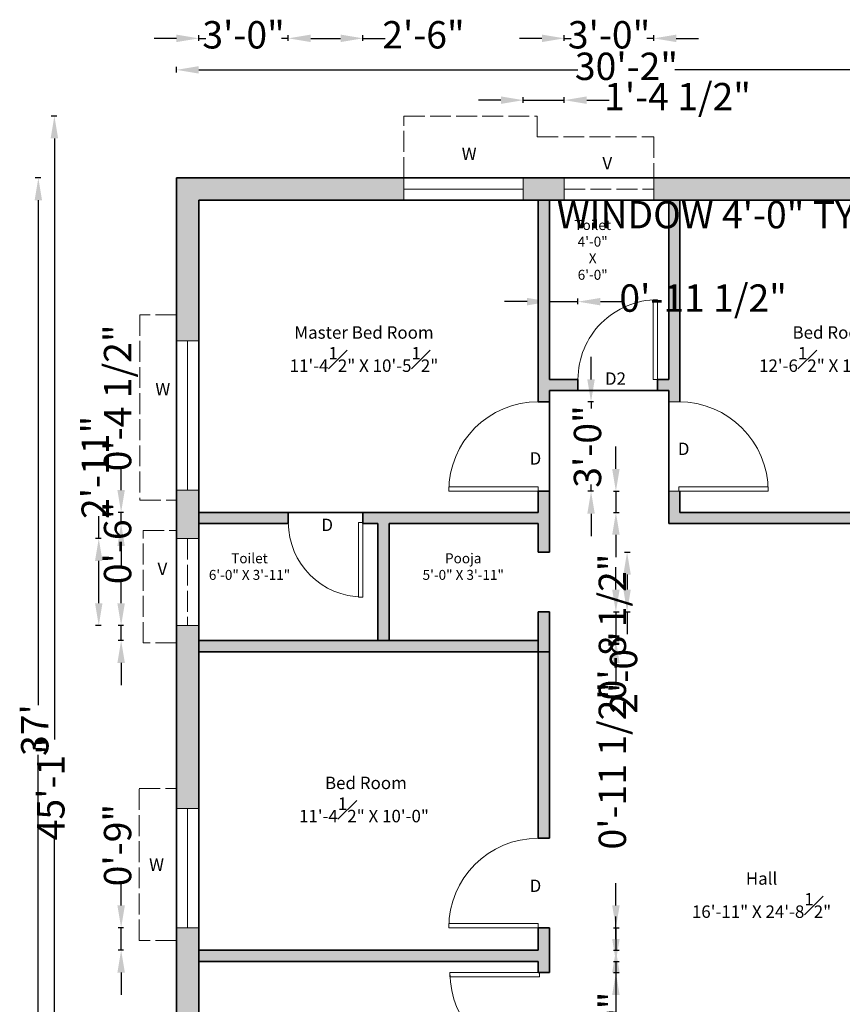
# Model space of a CAD drawing. Units: inches. Extents: x 2339 to 2848, y 489 to 1121.
# Tile 2 of 3: x 2339 to 2670, y 725 to 1121. Entities that reach past the tile are written whole.
import ezdxf

# ---------------------------------------------------------------- set-up
doc = ezdxf.new("R2010")
doc.units = ezdxf.units.IN
doc.linetypes.add('ACAD_ISO02W100', pattern=[15, 12, -3])
for name, color, linetype, lineweight in [('A-ANNO-DIMS', 2, 'Continuous', 18), ('A-ANNO-TEXT', 7, 'Continuous', 18), ('A-AREA-IDEN', 7, 'Continuous', 18), ('A-DOOR', 3, 'Continuous', 18), ('A-GLAZ', 4, 'Continuous', 18), ('A-GLAZ-VENT', 4, 'ACAD_ISO02W100', 18), ('A-ROOF-OVHD', 8, 'ACAD_ISO02W100', 13), ('A-WALL', 7, 'Continuous', 35)]:
    doc.layers.add(name, color=color, linetype=linetype, lineweight=lineweight)
doc.layers.add('A-WALL-PATT', color=18, linetype='Continuous', lineweight=13, true_color=0x000000)
doc.styles.get("Standard").update_dxf_attribs({"font": 'arial.ttf'})
doc.dimstyles.new('ISO-25', dxfattribs={"dimtxt": 11, "dimasz": 9, "dimexe": 1.25, "dimexo": 0.625, "dimtad": 0, "dimlunit": 4, "dimtxsty": 'Standard', "dimcen": 2.5, "dimadec": 0, "dimazin": 0, "dimtfac": 1, "dimtmove": 0, "dimatfit": 3, "dimfxl": 1, "dimfxlon": 1, "dimfrac": 1, "dimarcsym": 0})

# ---------------------------------------------------------------- blocks, each defined once
blk = doc.blocks.new('*U1')
for p, q in [((0, 0), (0, 4)), ((32, 0), (32, 4))]:
    blk.add_line(p, q)
blk.add_lwpolyline([(0, 0), (0, -32), (1.75, -32), (1.75, 0)], close=True)
blk.add_arc((0, 0), 32, 270, 0)
blk = doc.blocks.new('*U2')
for p, q in [((0, 0), (0, -4)), ((36, 0), (36, -4))]:
    blk.add_line(p, q)
blk.add_lwpolyline([(0, 0), (0, 36), (1.75, 36), (1.75, 0)], close=True)
blk.add_arc((0, 0), 36, 0, 90)
blk = doc.blocks.new('*U3')
for p, q in [((0, 0), (0, 4)), ((30, 0), (30, 4))]:
    blk.add_line(p, q)
blk.add_lwpolyline([(0, 0), (0, -30), (1.75, -30), (1.75, 0)], close=True)
blk.add_arc((0, 0), 30, 270, 0)
blk = doc.blocks.new('*D4')
at = {"layer": 'A-ANNO-DIMS', "color": 0, "lineweight": -2, "transparency": 16777216}
for p, q in [((2347.8, 1057.44), (2345.55, 1057.44)), ((2346.8, 1048.44), (2346.8, 845.39)), ((2346.8, 622.44), (2346.8, 825.48)), ((2347.8, 613.44), (2345.55, 613.44))]:
    blk.add_line(p, q, dxfattribs=at)
at = {"layer": 'A-ANNO-DIMS', "color": 0, "transparency": 16777216}
for points in [[(2345.3, 1048.44), (2348.3, 1048.44), (2346.8, 1057.44)], [(2345.3, 622.44), (2348.3, 622.44), (2346.8, 613.44)]]:
    blk.add_solid(points, dxfattribs=at)
at = {"layer": 'Defpoints', "color": 0, "transparency": 16777216}
for p in [(2402.35, 1057.44), (2346.8, 613.44), (2402.35, 613.44)]:
    blk.add_point(p, dxfattribs=at)
at = {"layer": 'A-ANNO-DIMS', "color": 0, "transparency": 16777216, "insert": (2346.8, 835.44), "char_height": 11, "attachment_point": 5, "rotation": 90}
blk.add_mtext("37'", dxfattribs=at)
blk = doc.blocks.new('*D6')
at = {"layer": 'A-ANNO-DIMS', "color": 0, "lineweight": -2, "transparency": 16777216}
for p, q in [((2402.35, 1099.88), (2402.35, 1102.13)), ((2411.35, 1100.88), (2563.83, 1100.88)), ((2755.35, 1100.88), (2602.86, 1100.88)), ((2764.35, 1099.88), (2764.35, 1102.13))]:
    blk.add_line(p, q, dxfattribs=at)
at = {"layer": 'A-ANNO-DIMS', "color": 0, "transparency": 16777216}
for points in [[(2411.35, 1102.38), (2411.35, 1099.38), (2402.35, 1100.88)], [(2755.35, 1102.38), (2755.35, 1099.38), (2764.35, 1100.88)]]:
    blk.add_solid(points, dxfattribs=at)
at = {"layer": 'Defpoints', "color": 0, "transparency": 16777216}
for p in [(2764.35, 1100.88), (2402.35, 1057.44), (2764.35, 1057.44)]:
    blk.add_point(p, dxfattribs=at)
at = {"layer": 'A-ANNO-DIMS', "color": 0, "transparency": 16777216, "insert": (2583.35, 1100.88), "char_height": 11, "attachment_point": 5}
blk.add_mtext('30\'-2"', dxfattribs=at)
blk = doc.blocks.new('WIN-48IN')
for p, q in [((0, 0), (0, 9)), ((48, 0), (48, 9)), ((0, 4.5), (48, 4.5))]:
    blk.add_line(p, q)
blk = doc.blocks.new('*D9')
at = {"layer": 'A-ANNO-DIMS', "color": 0, "lineweight": -2, "transparency": 16777216}
for p, q in [((2701.35, 1041.24), (2692.35, 1041.24)), ((2701.35, 1042.24), (2701.35, 1039.99)), ((2740.35, 1041.24), (2710.35, 1041.24)), ((2749.35, 1042.24), (2749.35, 1039.99))]:
    blk.add_line(p, q, dxfattribs=at)
at = {"layer": 'A-ANNO-DIMS', "color": 0, "transparency": 16777216}
for points in [[(2710.35, 1042.74), (2710.35, 1039.74), (2701.35, 1041.24)], [(2740.35, 1042.74), (2740.35, 1039.74), (2749.35, 1041.24)]]:
    blk.add_solid(points, dxfattribs=at)
at = {"layer": 'Defpoints', "color": 0, "transparency": 16777216}
for p in [(2701.35, 1048.44), (2749.35, 1048.44), (2701.35, 1041.24)]:
    blk.add_point(p, dxfattribs=at)
at = {"layer": 'A-ANNO-DIMS', "color": 0, "transparency": 16777216, "insert": (2622.12, 1041.24), "char_height": 11, "attachment_point": 5}
blk.add_mtext('WINDOW 4\'-0" TYP.', dxfattribs=at)
blk = doc.blocks.new('*D11')
at = {"layer": 'A-ANNO-DIMS', "color": 0, "lineweight": -2, "transparency": 16777216}
for p, q in [((2354.26, 1082.3), (2352.01, 1082.3)), ((2353.26, 1073.3), (2353.26, 831.61)), ((2353.26, 550.44), (2353.26, 792.13)), ((2354.26, 541.44), (2352.01, 541.44))]:
    blk.add_line(p, q, dxfattribs=at)
at = {"layer": 'A-ANNO-DIMS', "color": 0, "transparency": 16777216}
for points in [[(2351.76, 1073.3), (2354.76, 1073.3), (2353.26, 1082.3)], [(2351.76, 550.44), (2354.76, 550.44), (2353.26, 541.44)]]:
    blk.add_solid(points, dxfattribs=at)
at = {"layer": 'Defpoints', "color": 0, "transparency": 16777216}
for p in [(2353.26, 1082.3), (2493.85, 1082.3), (2402.35, 541.44)]:
    blk.add_point(p, dxfattribs=at)
at = {"layer": 'A-ANNO-DIMS', "color": 0, "transparency": 16777216, "insert": (2353.26, 811.87), "char_height": 11, "attachment_point": 5, "rotation": 90}
blk.add_mtext('45\'-1"', dxfattribs=at)
blk = doc.blocks.new('*D22')
at = {"layer": 'A-ANNO-DIMS', "color": 0, "lineweight": -2, "transparency": 16777216}
for p, q in [((2380.1, 764.94), (2380.1, 773.94)), ((2381.1, 755.94), (2378.85, 755.94)), ((2380.1, 746.94), (2380.1, 755.94)), ((2381.1, 746.94), (2378.85, 746.94)), ((2380.1, 737.94), (2380.1, 728.94))]:
    blk.add_line(p, q, dxfattribs=at)
at = {"layer": 'A-ANNO-DIMS', "color": 0, "transparency": 16777216}
for points in [[(2378.6, 764.94), (2381.6, 764.94), (2380.1, 755.94)], [(2378.6, 737.94), (2381.6, 737.94), (2380.1, 746.94)]]:
    blk.add_solid(points, dxfattribs=at)
at = {"layer": 'Defpoints', "color": 0, "transparency": 16777216}
for p in [(2380.1, 755.94), (2411.35, 755.94), (2411.35, 746.94)]:
    blk.add_point(p, dxfattribs=at)
at = {"layer": 'A-ANNO-DIMS', "color": 0, "transparency": 16777216, "insert": (2380.1, 789.18), "char_height": 11, "attachment_point": 5, "rotation": 90}
blk.add_mtext('0\'-9"', dxfattribs=at)
blk = doc.blocks.new('*D23')
at = {"layer": 'A-ANNO-DIMS', "color": 0, "lineweight": -2, "transparency": 16777216}
for p, q in [((2380.1, 886.44), (2380.1, 895.44)), ((2381.1, 877.44), (2378.85, 877.44)), ((2380.1, 871.44), (2380.1, 877.44)), ((2381.1, 871.44), (2378.85, 871.44)), ((2380.1, 862.44), (2380.1, 853.44))]:
    blk.add_line(p, q, dxfattribs=at)
at = {"layer": 'A-ANNO-DIMS', "color": 0, "transparency": 16777216}
for points in [[(2378.6, 886.44), (2381.6, 886.44), (2380.1, 877.44)], [(2378.6, 862.44), (2381.6, 862.44), (2380.1, 871.44)]]:
    blk.add_solid(points, dxfattribs=at)
at = {"layer": 'Defpoints', "color": 0, "transparency": 16777216}
for p in [(2380.1, 877.44), (2411.35, 877.44), (2411.35, 871.44)]:
    blk.add_point(p, dxfattribs=at)
at = {"layer": 'A-ANNO-DIMS', "color": 0, "transparency": 16777216, "insert": (2380.1, 910.68), "char_height": 11, "attachment_point": 5, "rotation": 90}
blk.add_mtext('0\'-6"', dxfattribs=at)
blk = doc.blocks.new('*D24')
at = {"layer": 'A-ANNO-DIMS', "color": 0, "lineweight": -2, "transparency": 16777216}
for p, q in [((2371.1, 912.44), (2371.1, 921.44)), ((2372.1, 912.44), (2369.85, 912.44)), ((2371.1, 886.44), (2371.1, 903.44)), ((2372.1, 877.44), (2369.85, 877.44))]:
    blk.add_line(p, q, dxfattribs=at)
at = {"layer": 'A-ANNO-DIMS', "color": 0, "transparency": 16777216}
for points in [[(2369.6, 903.44), (2372.6, 903.44), (2371.1, 912.44)], [(2369.6, 886.44), (2372.6, 886.44), (2371.1, 877.44)]]:
    blk.add_solid(points, dxfattribs=at)
at = {"layer": 'Defpoints', "color": 0, "transparency": 16777216}
for p in [(2371.1, 912.44), (2402.35, 912.44), (2402.35, 877.44)]:
    blk.add_point(p, dxfattribs=at)
at = {"layer": 'A-ANNO-DIMS', "color": 0, "transparency": 16777216, "insert": (2371.1, 941.05), "char_height": 11, "attachment_point": 5, "rotation": 90}
blk.add_mtext('2\'-11"', dxfattribs=at)
blk = doc.blocks.new('*D25')
at = {"layer": 'A-ANNO-DIMS', "color": 0, "lineweight": -2, "transparency": 16777216}
for p, q in [((2830.6, 991.94), (2832.85, 991.94)), ((2831.6, 982.94), (2831.6, 977.18)), ((2831.6, 940.94), (2831.6, 946.69)), ((2830.6, 931.94), (2832.85, 931.94))]:
    blk.add_line(p, q, dxfattribs=at)
at = {"layer": 'A-ANNO-DIMS', "color": 0, "transparency": 16777216}
for points in [[(2830.1, 982.94), (2833.1, 982.94), (2831.6, 991.94)], [(2830.1, 940.94), (2833.1, 940.94), (2831.6, 931.94)]]:
    blk.add_solid(points, dxfattribs=at)
at = {"layer": 'Defpoints', "color": 0, "transparency": 16777216}
for p in [(2411.35, 991.94), (2831.6, 991.94), (2411.35, 931.94)]:
    blk.add_point(p, dxfattribs=at)
at = {"layer": 'A-ANNO-DIMS', "color": 0, "transparency": 16777216, "insert": (2831.6, 961.94), "char_height": 11, "attachment_point": 5, "rotation": 90}
blk.add_mtext('5\'-0"', dxfattribs=at)
blk = doc.blocks.new('*D26')
at = {"layer": 'A-ANNO-DIMS', "color": 0, "lineweight": -2, "transparency": 16777216}
for p, q in [((2831.6, 1048.44), (2831.6, 1057.44)), ((2830.6, 1048.44), (2832.85, 1048.44)), ((2831.6, 1000.94), (2831.6, 1039.44)), ((2830.6, 991.94), (2832.85, 991.94))]:
    blk.add_line(p, q, dxfattribs=at)
at = {"layer": 'A-ANNO-DIMS', "color": 0, "transparency": 16777216}
for points in [[(2830.1, 1039.44), (2833.1, 1039.44), (2831.6, 1048.44)], [(2830.1, 1000.94), (2833.1, 1000.94), (2831.6, 991.94)]]:
    blk.add_solid(points, dxfattribs=at)
at = {"layer": 'Defpoints', "color": 0, "transparency": 16777216}
for p in [(2411.35, 1048.44), (2831.6, 1048.44), (2411.35, 991.94)]:
    blk.add_point(p, dxfattribs=at)
at = {"layer": 'A-ANNO-DIMS', "color": 0, "transparency": 16777216, "insert": (2831.6, 1085.72), "char_height": 11, "attachment_point": 5, "rotation": 90}
blk.add_mtext('4\'-8 1/2"', dxfattribs=at)
blk = doc.blocks.new('*D27')
at = {"layer": 'A-ANNO-DIMS', "color": 0, "lineweight": -2, "transparency": 16777216}
for p, q in [((2411.35, 511.19), (2411.35, 508.94)), ((2493.85, 511.19), (2493.85, 508.94)), ((2402.35, 510.19), (2393.35, 510.19)), ((2411.35, 510.19), (2420.23, 510.19)), ((2493.85, 510.19), (2484.96, 510.19)), ((2502.85, 510.19), (2511.85, 510.19))]:
    blk.add_line(p, q, dxfattribs=at)
at = {"layer": 'A-ANNO-DIMS', "color": 0, "transparency": 16777216}
for points in [[(2402.35, 511.69), (2402.35, 508.69), (2411.35, 510.19)], [(2502.85, 511.69), (2502.85, 508.69), (2493.85, 510.19)]]:
    blk.add_solid(points, dxfattribs=at)
at = {"layer": 'Defpoints', "color": 0, "transparency": 16777216}
for p in [(2411.35, 1048.44), (2493.85, 1048.44), (2493.85, 510.19)]:
    blk.add_point(p, dxfattribs=at)
at = {"layer": 'A-ANNO-DIMS', "color": 0, "transparency": 16777216, "insert": (2452.6, 510.19), "char_height": 11, "attachment_point": 5}
blk.add_mtext('6\'-10 1/2"', dxfattribs=at)
blk = doc.blocks.new('*D28')
at = {"layer": 'A-ANNO-DIMS', "color": 0, "lineweight": -2, "transparency": 16777216}
for p, q in [((2549.35, 1113.55), (2540.35, 1113.55)), ((2558.35, 1112.55), (2558.35, 1114.8)), ((2558.35, 1113.55), (2561.11, 1113.55)), ((2594.35, 1113.55), (2591.59, 1113.55)), ((2594.35, 1112.55), (2594.35, 1114.8)), ((2603.35, 1113.55), (2612.35, 1113.55))]:
    blk.add_line(p, q, dxfattribs=at)
at = {"layer": 'A-ANNO-DIMS', "color": 0, "transparency": 16777216}
for points in [[(2549.35, 1115.05), (2549.35, 1112.05), (2558.35, 1113.55)], [(2603.35, 1115.05), (2603.35, 1112.05), (2594.35, 1113.55)]]:
    blk.add_solid(points, dxfattribs=at)
at = {"layer": 'Defpoints', "color": 0, "transparency": 16777216}
for p in [(2594.35, 1113.55), (2558.35, 1057.44), (2594.35, 1057.44)]:
    blk.add_point(p, dxfattribs=at)
at = {"layer": 'A-ANNO-DIMS', "color": 0, "transparency": 16777216, "insert": (2576.35, 1113.55), "char_height": 11, "attachment_point": 5}
blk.add_mtext('3\'-0"', dxfattribs=at)
blk = doc.blocks.new('*D29')
at = {"layer": 'A-ANNO-DIMS', "color": 0, "lineweight": -2, "transparency": 16777216}
for p, q in [((2532.85, 1088.69), (2523.85, 1088.69)), ((2541.85, 1087.69), (2541.85, 1089.94)), ((2541.85, 1088.69), (2558.35, 1088.69)), ((2558.35, 1087.69), (2558.35, 1089.94)), ((2567.35, 1088.69), (2576.35, 1088.69))]:
    blk.add_line(p, q, dxfattribs=at)
at = {"layer": 'A-ANNO-DIMS', "color": 0, "transparency": 16777216}
for points in [[(2532.85, 1090.19), (2532.85, 1087.19), (2541.85, 1088.69)], [(2567.35, 1090.19), (2567.35, 1087.19), (2558.35, 1088.69)]]:
    blk.add_solid(points, dxfattribs=at)
at = {"layer": 'Defpoints', "color": 0, "transparency": 16777216}
for p in [(2558.35, 1088.69), (2541.85, 1057.44), (2558.35, 1057.44)]:
    blk.add_point(p, dxfattribs=at)
at = {"layer": 'A-ANNO-DIMS', "color": 0, "transparency": 16777216, "insert": (2603.89, 1088.69), "char_height": 11, "attachment_point": 5}
blk.add_mtext('1\'-4 1/2"', dxfattribs=at)
blk = doc.blocks.new('*D36')
at = {"layer": 'A-ANNO-DIMS', "color": 0, "lineweight": -2, "transparency": 16777216}
for p, q in [((2563.85, 511.19), (2563.85, 508.94)), ((2595.85, 511.19), (2595.85, 508.94)), ((2554.85, 510.19), (2545.85, 510.19)), ((2563.85, 510.19), (2564.51, 510.19)), ((2595.85, 510.19), (2595.19, 510.19)), ((2604.85, 510.19), (2613.85, 510.19))]:
    blk.add_line(p, q, dxfattribs=at)
at = {"layer": 'A-ANNO-DIMS', "color": 0, "transparency": 16777216}
for points in [[(2554.85, 511.69), (2554.85, 508.69), (2563.85, 510.19)], [(2604.85, 511.69), (2604.85, 508.69), (2595.85, 510.19)]]:
    blk.add_solid(points, dxfattribs=at)
at = {"layer": 'Defpoints', "color": 0, "transparency": 16777216}
for p in [(2563.85, 971.94), (2595.85, 971.94), (2595.85, 510.19)]:
    blk.add_point(p, dxfattribs=at)
at = {"layer": 'A-ANNO-DIMS', "color": 0, "transparency": 16777216, "insert": (2579.85, 510.19), "char_height": 11, "attachment_point": 5}
blk.add_mtext('2\'-8"', dxfattribs=at)
blk = doc.blocks.new('*D37')
at = {"layer": 'A-ANNO-DIMS', "color": 0, "lineweight": -2, "transparency": 16777216}
for p, q in [((2447.35, 1112.55), (2447.35, 1114.8)), ((2456.35, 1113.55), (2468.35, 1113.55)), ((2477.35, 1112.55), (2477.35, 1114.8)), ((2477.35, 1113.55), (2486.35, 1113.55))]:
    blk.add_line(p, q, dxfattribs=at)
at = {"layer": 'A-ANNO-DIMS', "color": 0, "transparency": 16777216}
for points in [[(2456.35, 1115.05), (2456.35, 1112.05), (2447.35, 1113.55)], [(2468.35, 1115.05), (2468.35, 1112.05), (2477.35, 1113.55)]]:
    blk.add_solid(points, dxfattribs=at)
at = {"layer": 'Defpoints', "color": 0, "transparency": 16777216}
for p in [(2477.35, 1113.55), (2447.35, 922.94), (2477.35, 922.94)]:
    blk.add_point(p, dxfattribs=at)
at = {"layer": 'A-ANNO-DIMS', "color": 0, "transparency": 16777216, "insert": (2501.69, 1113.55), "char_height": 11, "attachment_point": 5}
blk.add_mtext('2\'-6"', dxfattribs=at)
blk = doc.blocks.new('*D38')
at = {"layer": 'A-ANNO-DIMS', "color": 0, "lineweight": -2, "transparency": 16777216}
for p, q in [((2380.1, 931.94), (2380.1, 940.94)), ((2381.1, 922.94), (2378.85, 922.94)), ((2380.1, 918.44), (2380.1, 922.94)), ((2381.1, 918.44), (2378.85, 918.44)), ((2380.1, 909.44), (2380.1, 900.44))]:
    blk.add_line(p, q, dxfattribs=at)
at = {"layer": 'A-ANNO-DIMS', "color": 0, "transparency": 16777216}
for points in [[(2378.6, 931.94), (2381.6, 931.94), (2380.1, 922.94)], [(2378.6, 909.44), (2381.6, 909.44), (2380.1, 918.44)]]:
    blk.add_solid(points, dxfattribs=at)
at = {"layer": 'Defpoints', "color": 0, "transparency": 16777216}
for p in [(2380.1, 922.94), (2411.35, 922.94), (2411.35, 918.44)]:
    blk.add_point(p, dxfattribs=at)
at = {"layer": 'A-ANNO-DIMS', "color": 0, "transparency": 16777216, "insert": (2380.1, 969), "char_height": 11, "attachment_point": 5, "rotation": 90}
blk.add_mtext('0\'-4 1/2"', dxfattribs=at)
blk = doc.blocks.new('*D39')
at = {"layer": 'A-ANNO-DIMS', "color": 0, "lineweight": -2, "transparency": 16777216}
for p, q in [((2582.6, 906.94), (2584.85, 906.94)), ((2583.6, 897.94), (2583.6, 891.94)), ((2582.6, 882.94), (2584.85, 882.94)), ((2583.6, 882.94), (2583.6, 873.94))]:
    blk.add_line(p, q, dxfattribs=at)
at = {"layer": 'A-ANNO-DIMS', "color": 0, "transparency": 16777216}
for points in [[(2582.1, 897.94), (2585.1, 897.94), (2583.6, 906.94)], [(2582.1, 891.94), (2585.1, 891.94), (2583.6, 882.94)]]:
    blk.add_solid(points, dxfattribs=at)
at = {"layer": 'Defpoints', "color": 0, "transparency": 16777216}
for p in [(2552.35, 906.94), (2552.35, 882.94), (2583.6, 882.94)]:
    blk.add_point(p, dxfattribs=at)
at = {"layer": 'A-ANNO-DIMS', "color": 0, "transparency": 16777216, "insert": (2583.6, 858.6), "char_height": 11, "attachment_point": 5, "rotation": 90}
blk.add_mtext('2\'-0"', dxfattribs=at)
blk = doc.blocks.new('*D40')
at = {"layer": 'A-ANNO-DIMS', "color": 0, "lineweight": -2, "transparency": 16777216}
for p, q in [((2569.1, 976.44), (2569.1, 985.44)), ((2570.1, 967.44), (2567.85, 967.44)), ((2569.1, 967.44), (2569.1, 964.68)), ((2570.1, 931.44), (2567.85, 931.44)), ((2569.1, 931.44), (2569.1, 934.2)), ((2569.1, 922.44), (2569.1, 913.44))]:
    blk.add_line(p, q, dxfattribs=at)
at = {"layer": 'A-ANNO-DIMS', "color": 0, "transparency": 16777216}
for points in [[(2567.6, 976.44), (2570.6, 976.44), (2569.1, 967.44)], [(2567.6, 922.44), (2570.6, 922.44), (2569.1, 931.44)]]:
    blk.add_solid(points, dxfattribs=at)
at = {"layer": 'Defpoints', "color": 0, "transparency": 16777216}
for p in [(2569.1, 967.44), (2600.35, 967.44), (2600.35, 931.44)]:
    blk.add_point(p, dxfattribs=at)
at = {"layer": 'A-ANNO-DIMS', "color": 0, "transparency": 16777216, "insert": (2569.1, 949.44), "char_height": 11, "attachment_point": 5, "rotation": 90}
blk.add_mtext('3\'-0"', dxfattribs=at)
blk = doc.blocks.new('*D42')
at = {"layer": 'A-ANNO-DIMS', "color": 0, "lineweight": -2, "transparency": 16777216}
for p, q in [((2402.35, 1113.55), (2393.35, 1113.55)), ((2411.35, 1112.55), (2411.35, 1114.8)), ((2411.35, 1113.55), (2414.11, 1113.55)), ((2447.35, 1113.55), (2444.59, 1113.55)), ((2447.35, 1112.55), (2447.35, 1114.8)), ((2456.35, 1113.55), (2465.35, 1113.55))]:
    blk.add_line(p, q, dxfattribs=at)
at = {"layer": 'A-ANNO-DIMS', "color": 0, "transparency": 16777216}
for points in [[(2402.35, 1115.05), (2402.35, 1112.05), (2411.35, 1113.55)], [(2456.35, 1115.05), (2456.35, 1112.05), (2447.35, 1113.55)]]:
    blk.add_solid(points, dxfattribs=at)
at = {"layer": 'Defpoints', "color": 0, "transparency": 16777216}
for p in [(2447.35, 1113.55), (2411.35, 922.94), (2447.35, 922.94)]:
    blk.add_point(p, dxfattribs=at)
at = {"layer": 'A-ANNO-DIMS', "color": 0, "transparency": 16777216, "insert": (2429.35, 1113.55), "char_height": 11, "attachment_point": 5}
blk.add_mtext('3\'-0"', dxfattribs=at)
blk = doc.blocks.new('*D43')
at = {"layer": 'A-ANNO-DIMS', "color": 0, "lineweight": -2, "transparency": 16777216}
for p, q in [((2579.1, 940.44), (2579.1, 949.44)), ((2578.1, 931.44), (2580.35, 931.44)), ((2579.1, 931.44), (2579.1, 922.94)), ((2578.1, 922.94), (2580.35, 922.94)), ((2579.1, 913.94), (2579.1, 904.94))]:
    blk.add_line(p, q, dxfattribs=at)
at = {"layer": 'A-ANNO-DIMS', "color": 0, "transparency": 16777216}
for points in [[(2577.6, 940.44), (2580.6, 940.44), (2579.1, 931.44)], [(2577.6, 913.94), (2580.6, 913.94), (2579.1, 922.94)]]:
    blk.add_solid(points, dxfattribs=at)
at = {"layer": 'Defpoints', "color": 0, "transparency": 16777216}
for p in [(2547.85, 931.44), (2547.85, 922.94), (2579.1, 922.94)]:
    blk.add_point(p, dxfattribs=at)
at = {"layer": 'A-ANNO-DIMS', "color": 0, "transparency": 16777216, "insert": (2579.1, 876.88), "char_height": 11, "attachment_point": 5, "rotation": 90}
blk.add_mtext('0\'-8 1/2"', dxfattribs=at)
blk = doc.blocks.new('*D44')
at = {"layer": 'A-ANNO-DIMS', "color": 0, "lineweight": -2, "transparency": 16777216}
for p, q in [((2579.1, 891.94), (2579.1, 900.94)), ((2578.1, 882.94), (2580.35, 882.94)), ((2579.1, 882.94), (2579.1, 871.44)), ((2578.1, 871.44), (2580.35, 871.44)), ((2579.1, 862.44), (2579.1, 853.44))]:
    blk.add_line(p, q, dxfattribs=at)
at = {"layer": 'A-ANNO-DIMS', "color": 0, "transparency": 16777216}
for points in [[(2577.6, 891.94), (2580.6, 891.94), (2579.1, 882.94)], [(2577.6, 862.44), (2580.6, 862.44), (2579.1, 871.44)]]:
    blk.add_solid(points, dxfattribs=at)
at = {"layer": 'Defpoints', "color": 0, "transparency": 16777216}
for p in [(2547.85, 882.94), (2547.85, 871.44), (2579.1, 871.44)]:
    blk.add_point(p, dxfattribs=at)
at = {"layer": 'A-ANNO-DIMS', "color": 0, "transparency": 16777216, "insert": (2579.1, 821.1), "char_height": 11, "attachment_point": 5, "rotation": 90}
blk.add_mtext('0\'-11 1/2"', dxfattribs=at)
blk = doc.blocks.new('*D45')
at = {"layer": 'A-ANNO-DIMS', "color": 0, "lineweight": -2, "transparency": 16777216}
for p, q in [((2579.1, 764.94), (2579.1, 773.94)), ((2578.1, 755.94), (2580.35, 755.94)), ((2579.1, 755.94), (2579.1, 746.94)), ((2578.1, 746.94), (2580.35, 746.94)), ((2579.1, 737.94), (2579.1, 728.94))]:
    blk.add_line(p, q, dxfattribs=at)
at = {"layer": 'A-ANNO-DIMS', "color": 0, "transparency": 16777216}
for points in [[(2577.6, 764.94), (2580.6, 764.94), (2579.1, 755.94)], [(2577.6, 737.94), (2580.6, 737.94), (2579.1, 746.94)]]:
    blk.add_solid(points, dxfattribs=at)
at = {"layer": 'Defpoints', "color": 0, "transparency": 16777216}
for p in [(2547.85, 755.94), (2547.85, 746.94), (2579.1, 746.94)]:
    blk.add_point(p, dxfattribs=at)
at = {"layer": 'A-ANNO-DIMS', "color": 0, "transparency": 16777216, "insert": (2579.1, 713.69), "char_height": 11, "attachment_point": 5, "rotation": 90}
blk.add_mtext('0\'-9"', dxfattribs=at)
blk = doc.blocks.new('*D46')
at = {"layer": 'A-ANNO-DIMS', "color": 0, "lineweight": -2, "transparency": 16777216}
for p, q in [((2579.1, 751.44), (2579.1, 760.44)), ((2578.1, 742.44), (2580.35, 742.44)), ((2579.1, 742.44), (2579.1, 737.94)), ((2578.1, 737.94), (2580.35, 737.94)), ((2579.1, 728.94), (2579.1, 719.94))]:
    blk.add_line(p, q, dxfattribs=at)
at = {"layer": 'A-ANNO-DIMS', "color": 0, "transparency": 16777216}
for points in [[(2577.6, 751.44), (2580.6, 751.44), (2579.1, 742.44)], [(2577.6, 728.94), (2580.6, 728.94), (2579.1, 737.94)]]:
    blk.add_solid(points, dxfattribs=at)
at = {"layer": 'Defpoints', "color": 0, "transparency": 16777216}
for p in [(2547.85, 742.44), (2547.85, 737.94), (2579.1, 737.94)]:
    blk.add_point(p, dxfattribs=at)
at = {"layer": 'A-ANNO-DIMS', "color": 0, "transparency": 16777216, "insert": (2579.1, 691.88), "char_height": 11, "attachment_point": 5, "rotation": 90}
blk.add_mtext('0\'-4 1/2"', dxfattribs=at)
blk = doc.blocks.new('*D47')
at = {"layer": 'A-ANNO-DIMS', "color": 0, "lineweight": -2, "transparency": 16777216}
for p, q in [((2543.35, 1007.69), (2534.35, 1007.69)), ((2552.35, 1006.69), (2552.35, 1008.94)), ((2552.35, 1007.69), (2563.85, 1007.69)), ((2563.85, 1006.69), (2563.85, 1008.94)), ((2572.85, 1007.69), (2581.85, 1007.69))]:
    blk.add_line(p, q, dxfattribs=at)
at = {"layer": 'A-ANNO-DIMS', "color": 0, "transparency": 16777216}
for points in [[(2543.35, 1009.19), (2543.35, 1006.19), (2552.35, 1007.69)], [(2572.85, 1009.19), (2572.85, 1006.19), (2563.85, 1007.69)]]:
    blk.add_solid(points, dxfattribs=at)
at = {"layer": 'Defpoints', "color": 0, "transparency": 16777216}
for p in [(2563.85, 1007.69), (2552.35, 976.44), (2563.85, 976.44)]:
    blk.add_point(p, dxfattribs=at)
at = {"layer": 'A-ANNO-DIMS', "color": 0, "transparency": 16777216, "insert": (2614.18, 1007.69), "char_height": 11, "attachment_point": 5}
blk.add_mtext('0\'-11 1/2"', dxfattribs=at)

msp = doc.modelspace()

# ---------------------------------------------------------------- hatches: boundary and pattern name
at = {"layer": 'A-WALL-PATT'}
h = msp.add_hatch(color=256, dxfattribs=at)
h.dxf.hatch_style = 1
h.paths.add_polyline_path([(2493.847, 1057.438), (2402.347, 1057.438), (2402.347, 991.938), (2411.347, 991.938), (2411.347, 1048.438), (2493.847, 1048.438)])
h.paths.add_polyline_path([(2411.347, 931.938), (2402.347, 931.938), (2402.347, 912.438), (2411.347, 912.438), (2411.347, 918.438)])
h.paths.add_polyline_path([(2411.347, 871.438), (2411.347, 877.438), (2402.347, 877.438), (2402.347, 803.938), (2411.347, 803.938)])
h.paths.add_polyline_path([(2547.847, 871.438), (2411.347, 871.438), (2411.347, 866.938), (2547.847, 866.938)])
h.paths.add_polyline_path([(2447.347, 922.938), (2411.347, 922.938), (2411.347, 918.438), (2447.347, 918.438)])
h.paths.add_polyline_path([(2552.347, 866.938), (2547.847, 866.938), (2547.847, 791.938), (2552.347, 791.938)])
h.paths.add_polyline_path([(2411.347, 755.938), (2402.347, 755.938), (2402.347, 670.438), (2411.347, 670.438)])
h.paths.add_polyline_path([(2552.347, 755.938), (2547.847, 755.938), (2547.847, 746.938), (2411.347, 746.938), (2411.347, 742.438), (2547.847, 742.438), (2547.847, 737.938), (2552.347, 737.938)])
h.paths.add_polyline_path([(2552.347, 701.938), (2547.847, 701.938), (2547.847, 622.438), (2552.347, 622.438)])
h.paths.add_polyline_path([(2581.347, 622.438), (2411.347, 622.438), (2411.347, 634.438), (2402.347, 634.438), (2402.347, 613.438), (2581.347, 613.438)])
h.paths.add_polyline_path([(2695.347, 622.438), (2635.347, 622.438), (2635.347, 613.438), (2695.347, 613.438)])
h.paths.add_polyline_path([(2764.347, 628.438), (2755.347, 628.438), (2755.347, 622.438), (2749.347, 622.438), (2749.347, 613.438), (2764.347, 613.438)])
h.paths.add_polyline_path([(2764.347, 755.938), (2760.347, 755.938), (2755.347, 755.938), (2755.347, 676.438), (2764.347, 676.438)])
h.paths.add_polyline_path([(2764.347, 931.938), (2755.347, 931.938), (2755.347, 851.938), (2764.347, 851.938)])
h.paths.add_polyline_path([(2764.347, 1057.438), (2749.347, 1057.438), (2749.347, 1048.438), (2755.347, 1048.438), (2755.347, 979.938), (2764.347, 979.938)])
h.paths.add_polyline_path([(2701.347, 1057.438), (2594.347, 1057.438), (2594.347, 1048.438), (2604.847, 1048.438), (2701.347, 1048.438)])
h.paths.add_polyline_path([(2558.347, 1057.438), (2541.847, 1057.438), (2541.847, 1048.438), (2552.347, 1048.438), (2558.347, 1048.438)])
h = msp.add_hatch(color=256, dxfattribs=at)
h.dxf.hatch_style = 1
h.paths.add_polyline_path([(2552.347, 1048.438), (2547.847, 1048.438), (2547.847, 967.438), (2551.847, 967.438), (2552.347, 967.438), (2552.347, 971.938), (2563.847, 971.938), (2563.847, 976.438), (2552.347, 976.438)])
h.paths.add_polyline_path([(2604.847, 1048.438), (2600.347, 1048.438), (2600.347, 976.438), (2595.847, 976.438), (2595.847, 972.438), (2595.847, 971.938), (2600.347, 971.938), (2600.347, 967.438), (2604.347, 967.438, -0.0034723), (2604.847, 967.434)])
h.paths.add_polyline_path([(2604.847, 922.938), (2604.847, 931.438), (2604.347, 931.438), (2600.347, 931.438), (2600.347, 918.438), (2755.347, 918.438), (2755.347, 922.938)])
h = msp.add_hatch(color=256, dxfattribs=at)
h.dxf.hatch_style = 1
h.paths.add_polyline_path([(2487.847, 918.438), (2547.847, 918.438), (2547.847, 906.938), (2552.347, 906.938), (2552.347, 931.438), (2547.847, 931.438), (2547.847, 922.938), (2477.347, 922.938), (2477.347, 918.938), (2477.347, 918.438), (2483.347, 918.438), (2483.347, 871.438), (2487.847, 871.438)])
h.paths.add_polyline_path([(2552.347, 882.938), (2547.847, 882.938), (2547.847, 866.938), (2552.347, 866.938)])

# ---------------------------------------------------------------- linework, layer by layer
at = {"layer": 'A-GLAZ'}
for p, q in [((2558.347, 1048.438), (2558.347, 1057.438)), ((2594.347, 1048.438), (2594.347, 1057.438)), ((2411.347, 991.938), (2402.347, 991.938)), ((2406.847, 931.938), (2406.847, 991.938)), ((2411.347, 931.938), (2402.347, 931.938)), ((2411.347, 912.438), (2402.347, 912.438)), ((2411.347, 877.438), (2402.347, 877.438))]:
    msp.add_line(p, q, dxfattribs=at)
at = {"layer": 'A-GLAZ-VENT', "ltscale": 0.7}
for p, q in [((2558.347, 1052.938), (2594.347, 1052.938)), ((2406.847, 912.438), (2406.847, 877.438))]:
    msp.add_line(p, q, dxfattribs=at)
at = {"layer": 'A-ROOF-OVHD', "ltscale": 0.7}
for p, q in [((2493.847, 1057.438), (2493.847, 1082.304)), ((2493.847, 1082.304), (2547.486, 1082.304)), ((2547.486, 1082.304), (2547.486, 1073.929)), ((2547.486, 1073.929), (2594.347, 1073.929)), ((2594.347, 1073.929), (2594.347, 1057.438)), ((2402.347, 1002.378), (2387.676, 1002.378)), ((2387.676, 1002.378), (2387.676, 927.928)), ((2387.676, 927.928), (2402.347, 927.928)), ((2388.961, 870.486), (2388.961, 915.734)), ((2388.961, 915.734), (2402.347, 915.734)), ((2402.347, 870.486), (2388.961, 870.486)), ((2387.404, 750.844), (2387.404, 811.949)), ((2387.404, 811.949), (2402.347, 811.949)), ((2402.347, 750.844), (2387.404, 750.844))]:
    msp.add_line(p, q, dxfattribs=at)
at = {"layer": 'A-WALL'}
for p, q in [((2764.347, 1057.438), (2402.347, 1057.438)), ((2402.347, 1057.438), (2402.347, 613.438)), ((2411.347, 1048.438), (2411.347, 918.438)), ((2552.347, 1048.438), (2411.347, 1048.438)), ((2547.847, 1048.438), (2547.847, 967.438)), ((2552.347, 1048.438), (2552.347, 976.438)), ((2604.847, 1048.438), (2552.347, 1048.438)), ((2600.347, 1048.438), (2600.347, 976.438)), ((2755.347, 1048.438), (2604.847, 1048.438)), ((2604.847, 1048.438), (2604.847, 967.434)), ((2563.847, 976.438), (2552.347, 976.438)), ((2563.847, 976.438), (2563.847, 971.938)), ((2600.347, 976.438), (2595.847, 976.438)), ((2595.847, 971.938), (2595.847, 976.438)), ((2563.847, 971.938), (2552.347, 971.938)), ((2552.347, 971.938), (2552.347, 967.438)), ((2600.347, 971.938), (2563.847, 971.938)), ((2600.347, 971.938), (2600.347, 967.438)), ((2552.347, 967.438), (2547.847, 967.438)), ((2552.347, 967.438), (2552.347, 906.938)), ((2600.347, 967.438), (2600.347, 918.438)), ((2552.347, 931.438), (2547.847, 931.438)), ((2547.847, 931.438), (2547.847, 922.938)), ((2604.847, 931.438), (2604.847, 922.938)), ((2447.347, 922.938), (2411.347, 922.938)), ((2547.847, 922.938), (2447.347, 922.938)), ((2447.347, 922.938), (2447.347, 918.438)), ((2477.347, 922.938), (2477.347, 918.438)), ((2755.347, 922.938), (2604.847, 922.938)), ((2411.347, 918.438), (2411.347, 871.438)), ((2447.347, 918.438), (2411.347, 918.438)), ((2483.347, 918.438), (2477.347, 918.438)), ((2483.347, 918.438), (2483.347, 871.438)), ((2547.847, 918.438), (2487.847, 918.438)), ((2487.847, 918.438), (2487.847, 871.438)), ((2547.847, 918.438), (2547.847, 906.938)), ((2755.347, 918.438), (2600.347, 918.438)), ((2552.347, 906.938), (2547.847, 906.938)), ((2552.347, 882.938), (2547.847, 882.938)), ((2547.847, 882.938), (2547.847, 791.938)), ((2552.347, 882.938), (2552.347, 791.938)), ((2411.347, 871.438), (2411.347, 622.438)), ((2547.847, 871.438), (2411.347, 871.438)), ((2552.347, 866.938), (2411.347, 866.938)), ((2552.347, 791.938), (2547.847, 791.938)), ((2552.347, 755.938), (2547.847, 755.938)), ((2547.847, 755.938), (2547.847, 746.938)), ((2552.347, 755.938), (2552.347, 737.938)), ((2547.847, 746.938), (2411.347, 746.938)), ((2547.847, 742.438), (2411.347, 742.438)), ((2547.847, 742.438), (2547.847, 737.938)), ((2547.847, 737.938), (2552.347, 737.938))]:
    msp.add_line(p, q, dxfattribs=at)

# ---------------------------------------------------------------- block references
at = {"layer": 'A-DOOR'}
for name, p, rotation in [('*U1', (2595.847, 976.438), 180), ('*U2', (2547.847, 931.438), 90), ('*U2', (2547.847, 755.938), 90)]:
    msp.add_blockref(name, p, dxfattribs=dict(at, rotation=rotation))
at = {"layer": 'A-DOOR', "xscale": -1}
for p, rotation in [((2604.347, 931.438), 270), ((2548.347, 737.938), 90)]:
    msp.add_blockref('*U2', p, dxfattribs=dict(at, rotation=rotation))
msp.add_blockref('*U3', (2477.347, 918.938), dxfattribs=at)
at = {"layer": 'A-GLAZ'}
msp.add_blockref('WIN-48IN', (2493.847, 1048.438), dxfattribs=at)
at = {"layer": 'A-GLAZ', "rotation": 269.9999999999995}
msp.add_blockref('WIN-48IN', (2402.347, 803.938), dxfattribs=at)

# ---------------------------------------------------------------- texts
at = {"layer": 'A-ANNO-TEXT', "ltscale": 0.7, "char_height": 5, "attachment_point": 1}
for s, insert in [('\\pxqc;W', (2512.956, 1069.628)), ('\\pxqc;V', (2568.517, 1065.825)), ('\\pxqc;W', (2387.23, 783.835))]:
    msp.add_mtext_dynamic_manual_height_columns(s, width=14.23587, gutter_width=12.5, heights=[0], dxfattribs=dict(at, insert=insert))
at = {"layer": 'A-ANNO-TEXT', "char_height": 5, "attachment_point": 1}
for s, insert in [('\\pxqc;D2', (2571.802, 979.254)), ('\\pxqc;W', (2389.75, 974.994)), ('\\pxqc;D', (2599.227, 951.005)), ('\\pxqc;D', (2539.621, 947.155)), ('\\pxqc;D', (2455.876, 920.44)), ('\\pxqc;V', (2389.586, 902.729)), ('\\pxqc;D', (2539.621, 775.338))]:
    msp.add_mtext_dynamic_manual_height_columns(s, width=14.23587, gutter_width=12.5, heights=[0], dxfattribs=dict(at, insert=insert))
at = {"layer": 'A-AREA-IDEN', "attachment_point": 1}
for s, width, insert, char_height in [('\\pxqc;Toilet\\P4\'-0"\\PX\\P6\'-0"', 20.99649, (2559.262, 1040.489), 4), ('\\pxqc;Master Bed Room\\P11\'-4\\S1#2;" X 10\'-5\\S1#2;"', 97.24493, (2429.155, 997.789), 5), ('\\pxqc;Bed Room\\P12\'-6\\S1#2;" X 10\'-5\\S1#2;"', 97.24493, (2617.965, 997.789), 5), ('\\pxqc;Toilet\\P6\'-0" X 3\'-11"', 34.91256, (2414.28, 906.503), 4), ('\\pxqc;Pooja\\P5\'-0" X 3\'-11"', 34.91256, (2500.246, 906.503), 4), ('\\pxqc; Bed Room\\P11\'-4\\S1#2;" X 10\'-0"', 97.24493, (2429.155, 816.693), 5), ('\\pxqc;Hall\\P16\'-11" X 24\'-8\\S1#2;"', 97.24493, (2589.058, 778.269), 5)]:
    msp.add_mtext_dynamic_manual_height_columns(s, width=width, gutter_width=12.5, heights=[0], dxfattribs=dict(at, insert=insert, char_height=char_height))

# ---------------------------------------------------------------- dimensions: what is measured, and where the dimension line sits
at = {"layer": 'A-ANNO-DIMS'}
for base, p1, p2, override, picture, middle in [((2447.347, 1113.554), (2411.347, 922.938), (2447.347, 922.938), {"dimdec": 1, "dimlfac": 1, "dimrnd": 0, "dimzin": 1, "dimdsep": 46, "dimlunit": 4, "dimfrac": 2}, '*D42', (2429.347, 1113.554)), ((2477.347, 1113.554), (2447.347, 922.938), (2477.347, 922.938), {"dimdec": 1, "dimlfac": 1, "dimrnd": 0, "dimzin": 1, "dimdsep": 46, "dimlunit": 4, "dimfrac": 2}, '*D37', (2501.686, 1113.554)), ((2594.347, 1113.554), (2558.347, 1057.438), (2594.347, 1057.438), {"dimdec": 1, "dimlfac": 1, "dimrnd": 0, "dimzin": 1, "dimdsep": 46, "dimlunit": 4, "dimfrac": 2}, '*D28', (2576.347, 1113.554)), ((2764.347, 1100.878), (2402.347, 1057.438), (2764.347, 1057.438), {"dimclrd": 0, "dimclre": 0, "dimclrt": 0}, '*D6', (2583.347, 1100.878)), ((2558.347, 1088.688), (2541.847, 1057.438), (2558.347, 1057.438), {"dimdec": 1, "dimlfac": 1, "dimrnd": 0, "dimzin": 1, "dimdsep": 46, "dimlunit": 4, "dimfrac": 2}, '*D29', (2603.89, 1088.688)), ((2493.847, 510.188), (2411.347, 1048.438), (2493.847, 1048.438), {"dimdec": 1, "dimlfac": 1, "dimrnd": 0, "dimzin": 1, "dimdsep": 46, "dimlunit": 4, "dimfrac": 2}, '*D27', (2452.597, 510.188)), ((2563.847, 1007.688), (2552.347, 976.438), (2563.847, 976.438), {"dimdec": 1, "dimlfac": 1, "dimrnd": 0, "dimzin": 1, "dimdsep": 46, "dimlunit": 4, "dimfrac": 2}, '*D47', (2614.181, 1007.688)), ((2595.847, 510.188), (2563.847, 971.938), (2595.847, 971.938), {"dimdec": 1, "dimlfac": 1, "dimrnd": 0, "dimzin": 1, "dimdsep": 46, "dimlunit": 4, "dimfrac": 2}, '*D36', (2579.847, 510.188))]:
    dim = msp.add_linear_dim(base=base, p1=p1, p2=p2, dimstyle='ISO-25', override=override, dxfattribs=at)
    dim.commit()
    dim.dimension.update_dxf_attribs({"geometry": picture, "text_midpoint": middle})
for base, p1, p2, angle, override, picture, middle in [((2831.597, 1048.438), (2411.347, 991.938), (2411.347, 1048.438), 90, {"dimdec": 1, "dimlfac": 1, "dimrnd": 0, "dimzin": 1, "dimdsep": 46, "dimlunit": 4, "dimfrac": 2}, '*D26', (2831.597, 1085.72)), ((2353.26, 1082.304), (2402.347, 541.438), (2493.847, 1082.304), 90, {"dimdec": 1, "dimlfac": 1, "dimrnd": 0, "dimzin": 1, "dimdsep": 46, "dimlunit": 4, "dimfrac": 2}, '*D11', (2353.26, 811.871)), ((2346.8, 613.438), (2402.347, 1057.438), (2402.347, 613.438), 90, {"dimclrd": 0, "dimclre": 0, "dimclrt": 0}, '*D4', (2346.8, 835.438)), ((2380.097, 922.938), (2411.347, 918.438), (2411.347, 922.938), 90, {"dimdec": 1, "dimlfac": 1, "dimrnd": 0, "dimzin": 1, "dimdsep": 46, "dimlunit": 4, "dimfrac": 2}, '*D38', (2380.097, 968.999)), ((2831.597, 991.938), (2411.347, 931.938), (2411.347, 991.938), 90, {"dimdec": 1, "dimlfac": 1, "dimrnd": 0, "dimzin": 1, "dimdsep": 46, "dimlunit": 4, "dimfrac": 2}, '*D25', (2831.597, 961.938)), ((2569.097, 967.438), (2600.347, 931.438), (2600.347, 967.438), 90, {"dimdec": 1, "dimlfac": 1, "dimrnd": 0, "dimzin": 1, "dimdsep": 46, "dimlunit": 4, "dimfrac": 2}, '*D40', (2569.097, 949.438)), ((2371.097, 912.438), (2402.347, 877.438), (2402.347, 912.438), 90, {"dimdec": 1, "dimlfac": 1, "dimrnd": 0, "dimzin": 1, "dimdsep": 46, "dimlunit": 4, "dimfrac": 2}, '*D24', (2371.097, 941.05)), ((2579.097, 922.938), (2547.847, 931.438), (2547.847, 922.938), 270, {"dimdec": 1, "dimlfac": 1, "dimrnd": 0, "dimzin": 1, "dimdsep": 46, "dimlunit": 4, "dimfrac": 2}, '*D43', (2579.097, 876.876)), ((2380.097, 877.438), (2411.347, 871.438), (2411.347, 877.438), 90, {"dimdec": 1, "dimlfac": 1, "dimrnd": 0, "dimzin": 1, "dimdsep": 46, "dimlunit": 4, "dimfrac": 2}, '*D23', (2380.097, 910.683)), ((2583.597, 882.938), (2552.347, 906.938), (2552.347, 882.938), 270, {"dimdec": 1, "dimlfac": 1, "dimrnd": 0, "dimzin": 1, "dimdsep": 46, "dimlunit": 4, "dimfrac": 2}, '*D39', (2583.597, 858.599)), ((2579.097, 871.438), (2547.847, 882.938), (2547.847, 871.438), 270, {"dimdec": 1, "dimlfac": 1, "dimrnd": 0, "dimzin": 1, "dimdsep": 46, "dimlunit": 4, "dimfrac": 2}, '*D44', (2579.097, 821.103)), ((2380.097, 755.938), (2411.347, 746.938), (2411.347, 755.938), 90, {"dimdec": 1, "dimlfac": 1, "dimrnd": 0, "dimzin": 1, "dimdsep": 46, "dimlunit": 4, "dimfrac": 2}, '*D22', (2380.097, 789.183)), ((2579.097, 746.938), (2547.847, 755.938), (2547.847, 746.938), 270, {"dimdec": 1, "dimlfac": 1, "dimrnd": 0, "dimzin": 1, "dimdsep": 46, "dimlunit": 4, "dimfrac": 2}, '*D45', (2579.097, 713.692)), ((2579.097, 737.938), (2547.847, 742.438), (2547.847, 737.938), 270, {"dimdec": 1, "dimlfac": 1, "dimrnd": 0, "dimzin": 1, "dimdsep": 46, "dimlunit": 4, "dimfrac": 2}, '*D46', (2579.097, 691.876))]:
    dim = msp.add_linear_dim(base=base, p1=p1, p2=p2, angle=angle, dimstyle='ISO-25', override=override, dxfattribs=at)
    dim.commit()
    dim.dimension.update_dxf_attribs({"geometry": picture, "text_midpoint": middle})
dim = msp.add_linear_dim(base=(2701.347, 1041.238), p1=(2749.347, 1048.438), p2=(2701.347, 1048.438), angle=180, text='WINDOW <> TYP.', dimstyle='ISO-25', override={"dimdec": 1, "dimlfac": 1, "dimrnd": 0, "dimzin": 1, "dimdsep": 46, "dimlunit": 4, "dimfrac": 2}, dxfattribs=at)
dim.commit()
dim.dimension.update_dxf_attribs({"geometry": '*D9', "text_midpoint": (2622.124, 1041.238)})

doc.saveas('drawing.dxf')
